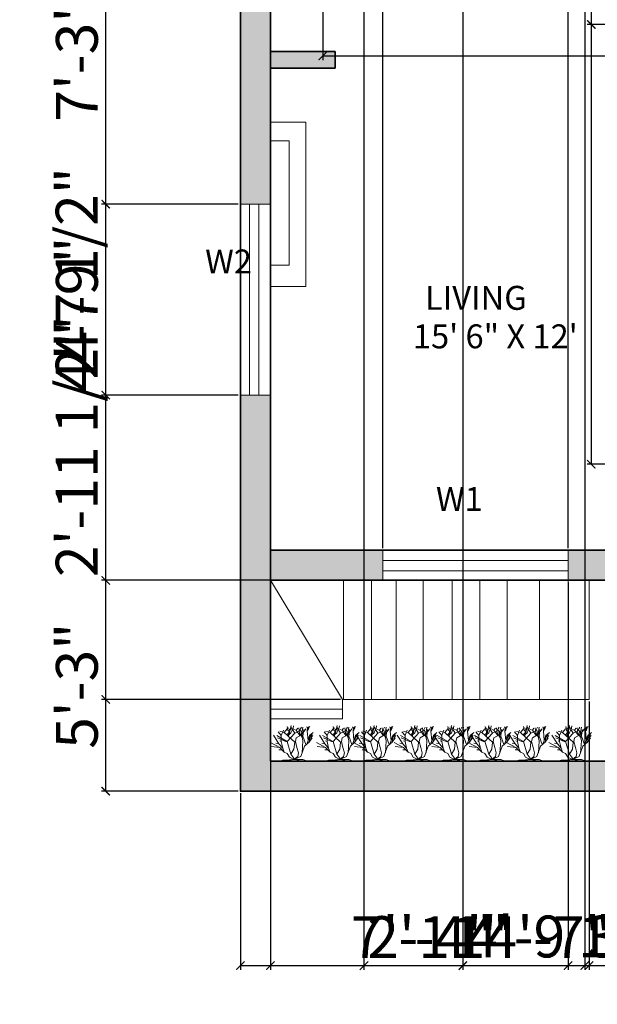
# Model space of a CAD drawing. Units: inches. Extents: x 1763 to 2368, y 1500 to 2097.
# Tile 1 of 24: x 1763 to 1936, y 1500 to 1794. Entities that reach past the tile are written whole.
import ezdxf

# ---------------------------------------------------------------- set-up
doc = ezdxf.new("R2010")
doc.units = ezdxf.units.IN
for name, color, linetype, lineweight in [('A-ANNO-DIMS', 2, 'Continuous', 18), ('A-ANNO-TEXT', 7, 'Continuous', 18), ('A-AREA-IDEN', 7, 'Continuous', 18), ('A-FLOR-STRS', 7, 'Continuous', 18), ('A-FURN', 8, 'Continuous', 18), ('A-WALL', 7, 'Continuous', 35), ('A-WALL-PATT', 7, 'Continuous', 13), ('trees', 3, 'Continuous', 13), ('windows', 1, 'Continuous', 18)]:
    doc.layers.add(name, color=color, linetype=linetype, lineweight=lineweight)
doc.styles.get("Standard").update_dxf_attribs({"font": 'arial.ttf'})
doc.dimstyles.new('ISO-25', dxfattribs={"dimtxt": 12.5, "dimasz": 2.5, "dimexe": 1.25, "dimexo": 0.625, "dimtad": 1, "dimdec": 0, "dimlunit": 4, "dimtxsty": 'Standard', "dimblk": 'ARCHTICK', "dimcen": 2.5, "dimclrd": 3, "dimclrt": 4, "dimadec": 0, "dimazin": 0, "dimtfac": 1, "dimtdec": 0, "dimtmove": 0, "dimatfit": 3, "dimfxl": 1, "dimarcsym": 0})

# ---------------------------------------------------------------- blocks, each defined once
blk = doc.blocks.new('*U17')
for p, q in [((-14.88, 18.24), (-17.76, 19.2)), ((-16.8, 16.32), (-15.36, 19.68)), ((-14.88, 18.24), (-12.96, 20.64)), ((-12.471, 19.775), (-12.898, 22.044)), ((-11.677, 19.071), (-12.471, 19.775)), ((-11.28, 19.619), (-12.104, 21.184)), ((-11.921, 18.836), (-10.64, 20.401)), ((-11.433, 18.289), (-10.457, 22.749)), ((-10.579, 18.054), (-9.846, 19.697)), ((-8.16, 17.76), (-10.56, 21.6)), ((-9.48, 19.775), (-8.992, 22.592)), ((-7.2, 19.68), (-8.64, 20.16)), ((-8.16, 17.76), (-5.28, 19.2)), ((-7.2, 19.68), (-6.24, 21.12)), ((-4.8, 16.32), (-7.2, 19.68)), ((-5.086, 17.741), (-5.513, 21.34)), ((-5.28, 19.2), (-3.84, 21.6)), ((-2.88, 12.96), (-4.32, 19.68)), ((-3.84, 16.8), (-0.96, 20.64)), ((-3.377, 18.602), (-2.888, 21.575)), ((-2.88, 15.84), (-2.4, 20.16)), ((-0.508, 21.888), (-0.081, 20.558)), ((-0.203, 19.149), (0.102, 21.34)), ((0.346, 13.203), (-0.203, 19.149)), ((-0.142, 19.384), (0.59, 20.401)), ((-0.02, 20.01), (0.896, 21.105)), ((0.041, 20.714), (1.384, 22.044)), ((0.102, 21.34), (0.835, 21.888)), ((-18.24, 11.04), (-21.755, 16.655)), ((-12.96, 12.48), (-19.68, 16.32)), ((-13.92, 12.48), (-19.2, 14.88)), ((-16.8, 16.32), (-18.72, 18.72)), ((-16.8, 12.48), (-17.76, 12.96)), ((-16.8, 12.48), (-16.8, 16.32)), ((-8.16, 12), (-14.88, 18.24)), ((-13.325, 16.724), (-11.433, 18.289)), ((-12.96, 12.48), (-8.16, 17.76)), ((-12.043, 15.628), (-11.921, 18.836)), ((-11.982, 16.802), (-10.579, 18.054)), ((-7.68, 12.48), (-7.2, 14.88)), ((-7.2, 14.88), (-3.84, 16.8)), ((-3.377, 15.315), (-5.086, 17.819)), ((-2.766, 16.802), (-3.377, 18.602)), ((-3.36, 5.28), (-2.88, 12.96)), ((-0.96, 10.56), (-2.88, 15.84)), ((-0.48, 10.8), (0.346, 13.203)), ((0.346, 13.203), (1.323, 16.254)), ((0.96, 12), (1.44, 15.36)), ((0.96, 12), (2.88, 14.88)), ((1.323, 16.254), (3.642, 18.289)), ((1.44, 15.36), (2.88, 17.28)), ((1.92, 13.44), (2.4, 15.36)), ((2.4, 15.36), (3.36, 16.32)), ((-17.76, 8.64), (-23.663, 11.961)), ((-17.76, 8.64), (-23.128, 9.222)), ((-18.24, 11.04), (-20.16, 11.52)), ((-15.84, 8.16), (-18.24, 11.04)), ((-16.32, 7.2), (-18.24, 7.2)), ((-14.88, 5.76), (-17.76, 8.64)), ((-15.84, 8.16), (-16.8, 12.48)), ((-14.88, 5.76), (-15.84, 8.16)), ((-12.96, 12.48), (-13.92, 12.48)), ((-10.56, 4.32), (-12.96, 12.48)), ((-10.56, 4.32), (-8.64, 7.68)), ((-8.64, 7.68), (-8.16, 12)), ((-6.72, 8.64), (-7.68, 12.48)), ((-5.76, 5.28), (-6.72, 8.64)), ((-4.32, 2.88), (-1.92, 9.6)), ((-1.92, 9.6), (0.96, 12)), ((-15.84, 0.48), (-17.76, 0)), ((-13.44, 0.48), (-15.84, 0.48)), ((-12.96, 4.8), (-14.88, 5.76)), ((-9.6, 0.96), (-13.44, 0.48)), ((-11.52, 2.4), (-12.96, 4.8)), ((-9.6, 0.96), (-12.96, 0)), ((-8.64, 0.96), (-11.52, 2.4)), ((-8.64, 1.92), (-10.56, 4.32)), ((-9.6, 0.96), (-7.68, 0.96)), ((-8.64, 0.96), (-4.32, 2.88)), ((-8.64, 0.96), (-6.24, 2.88)), ((-8.64, 0.96), (-8.64, 1.92)), ((-8.64, 0.96), (-2.88, 0.96)), ((-7.68, 0.96), (-6.24, 0.48)), ((-6.24, 2.88), (-5.76, 5.28)), ((-6.24, 0.48), (-3.36, 0)), ((-2.88, 0.96), (0, 0))]:
    blk.add_line(p, q)
blk = doc.blocks.new('_ArchTick')
at = {"color": 0, "linetype": 'ByBlock', "const_width": 0.15}
blk.add_lwpolyline([(-0.5, -0.5), (0.5, 0.5)], dxfattribs=at)
blk = doc.blocks.new('*D25')
at = {"layer": 'A-ANNO-DIMS', "color": 3, "lineweight": -2, "transparency": 16777216}
for p, q in [((1934.01, 1792.31), (1934.01, 1981.61)), ((1934.01, 1660.94), (1934.01, 1792.31))]:
    blk.add_line(p, q, dxfattribs=at)
at = {"layer": 'A-ANNO-DIMS', "color": 0, "lineweight": -2, "transparency": 16777216}
for p, q in [((1953.09, 1792.31), (1932.76, 1792.31)), ((1953.09, 1660.94), (1932.76, 1660.94))]:
    blk.add_line(p, q, dxfattribs=at)
at = {"layer": 'Defpoints', "color": 0, "transparency": 16777216}
for p in [(1934.01, 1792.31), (1953.72, 1792.31), (1953.72, 1660.94)]:
    blk.add_point(p, dxfattribs=at)
at = {"layer": 'A-ANNO-DIMS', "color": 3, "lineweight": -2, "transparency": 16777216, "xscale": 2.5, "yscale": 2.5, "zscale": 2.5}
for p, rotation in [((1934.01, 1792.31), 90), ((1934.01, 1660.94), 270)]:
    blk.add_blockref('_ArchTick', p, dxfattribs=dict(at, rotation=rotation))
at = {"layer": 'A-ANNO-DIMS', "color": 4, "transparency": 16777216, "insert": (1926.92, 1888.21), "char_height": 12.5, "attachment_point": 5, "rotation": 90}
blk.add_mtext('SECTIONAL 10\'-11 1/2"', dxfattribs=at)
blk = doc.blocks.new('*D27')
at = {"layer": 'A-ANNO-DIMS', "color": 0, "lineweight": -2, "transparency": 16777216}
for p, q in [((1853.71, 1795.96), (1853.71, 1781.68)), ((1944.71, 1795.96), (1944.71, 1781.68))]:
    blk.add_line(p, q, dxfattribs=at)
at = {"layer": 'A-ANNO-DIMS', "color": 3, "lineweight": -2, "transparency": 16777216}
for p, q in [((1853.71, 1782.93), (1944.71, 1782.93)), ((1944.71, 1782.93), (2085.85, 1782.93))]:
    blk.add_line(p, q, dxfattribs=at)
at = {"layer": 'Defpoints', "color": 0, "transparency": 16777216}
for p in [(1853.71, 1796.58), (1944.71, 1796.58), (1944.71, 1782.93)]:
    blk.add_point(p, dxfattribs=at)
at = {"layer": 'A-ANNO-DIMS', "color": 3, "lineweight": -2, "transparency": 16777216, "xscale": 2.5, "yscale": 2.5, "zscale": 2.5, "rotation": 180}
blk.add_blockref('_ArchTick', (1853.71, 1782.93), dxfattribs=at)
at = {"layer": 'A-ANNO-DIMS', "color": 3, "lineweight": -2, "transparency": 16777216, "xscale": 2.5, "yscale": 2.5, "zscale": 2.5}
blk.add_blockref('_ArchTick', (1944.71, 1782.93), dxfattribs=at)
at = {"layer": 'A-ANNO-DIMS', "color": 4, "transparency": 16777216, "insert": (2016.53, 1790.02), "char_height": 12.5, "attachment_point": 5}
blk.add_mtext('DINING SET 7\'-7"', dxfattribs=at)
blk = doc.blocks.new('*D39')
at = {"layer": 'A-ANNO-DIMS', "color": 0, "lineweight": -2, "transparency": 16777216}
for p, q in [((1829.09, 1562.65), (1829.09, 1509.91)), ((2003.86, 1562.65), (2003.86, 1509.91))]:
    blk.add_line(p, q, dxfattribs=at)
at = {"layer": 'A-ANNO-DIMS', "color": 3, "lineweight": -2, "transparency": 16777216}
blk.add_line((1829.09, 1511.16), (2003.86, 1511.16), dxfattribs=at)
at = {"layer": 'Defpoints', "color": 0, "transparency": 16777216}
for p in [(1829.09, 1563.27), (2003.86, 1563.27), (2003.86, 1511.16)]:
    blk.add_point(p, dxfattribs=at)
at = {"layer": 'A-ANNO-DIMS', "color": 3, "lineweight": -2, "transparency": 16777216, "xscale": 2.5, "yscale": 2.5, "zscale": 2.5, "rotation": 180}
blk.add_blockref('_ArchTick', (1829.09, 1511.16), dxfattribs=at)
at = {"layer": 'A-ANNO-DIMS', "color": 3, "lineweight": -2, "transparency": 16777216, "xscale": 2.5, "yscale": 2.5, "zscale": 2.5}
blk.add_blockref('_ArchTick', (2003.86, 1511.16), dxfattribs=at)
at = {"layer": 'A-ANNO-DIMS', "color": 4, "transparency": 16777216, "insert": (1916.48, 1518.06), "char_height": 12.5, "attachment_point": 5}
blk.add_mtext('14\'-7"', dxfattribs=at)
blk = doc.blocks.new('*D41')
at = {"layer": 'A-ANNO-DIMS', "color": 0, "lineweight": -2, "transparency": 16777216}
for p, q in [((1837.47, 1626.27), (1787.6, 1626.27)), ((1828.47, 1563.27), (1787.6, 1563.27))]:
    blk.add_line(p, q, dxfattribs=at)
at = {"layer": 'A-ANNO-DIMS', "color": 3, "lineweight": -2, "transparency": 16777216}
blk.add_line((1788.85, 1563.27), (1788.85, 1626.27), dxfattribs=at)
at = {"layer": 'Defpoints', "color": 0, "transparency": 16777216}
for p in [(1788.85, 1626.27), (1838.09, 1626.27), (1829.09, 1563.27)]:
    blk.add_point(p, dxfattribs=at)
at = {"layer": 'A-ANNO-DIMS', "color": 3, "lineweight": -2, "transparency": 16777216, "xscale": 2.5, "yscale": 2.5, "zscale": 2.5}
for p, rotation in [((1788.85, 1626.27), 90), ((1788.85, 1563.27), 270)]:
    blk.add_blockref('_ArchTick', p, dxfattribs=dict(at, rotation=rotation))
at = {"layer": 'A-ANNO-DIMS', "color": 4, "transparency": 16777216, "insert": (1781.84, 1594.77), "char_height": 12.5, "attachment_point": 5, "rotation": 90}
blk.add_mtext('5\'-3"', dxfattribs=at)
blk = doc.blocks.new('*D45')
at = {"layer": 'A-ANNO-DIMS', "color": 3, "lineweight": -2, "transparency": 16777216}
for p, q in [((1788.85, 1681.59), (1788.85, 1748.2)), ((1788.85, 1626.27), (1788.85, 1681.59))]:
    blk.add_line(p, q, dxfattribs=at)
at = {"layer": 'A-ANNO-DIMS', "color": 0, "lineweight": -2, "transparency": 16777216}
for p, q in [((1828.47, 1681.59), (1787.6, 1681.59)), ((1837.47, 1626.27), (1787.6, 1626.27))]:
    blk.add_line(p, q, dxfattribs=at)
at = {"layer": 'Defpoints', "color": 0, "transparency": 16777216}
for p in [(1788.85, 1681.59), (1829.09, 1681.59), (1838.09, 1626.27)]:
    blk.add_point(p, dxfattribs=at)
at = {"layer": 'A-ANNO-DIMS', "color": 3, "lineweight": -2, "transparency": 16777216, "xscale": 2.5, "yscale": 2.5, "zscale": 2.5}
for p, rotation in [((1788.85, 1681.59), 90), ((1788.85, 1626.27), 270)]:
    blk.add_blockref('_ArchTick', p, dxfattribs=dict(at, rotation=rotation))
at = {"layer": 'A-ANNO-DIMS', "color": 4, "transparency": 16777216, "insert": (1781.77, 1716.15), "char_height": 12.5, "attachment_point": 5, "rotation": 90}
blk.add_mtext('4\'-7 1/2"', dxfattribs=at)
blk = doc.blocks.new('*D46')
at = {"layer": 'A-ANNO-DIMS', "color": 0, "lineweight": -2, "transparency": 16777216}
for p, q in [((1828.47, 1738.64), (1787.6, 1738.64)), ((1828.47, 1681.59), (1787.6, 1681.59))]:
    blk.add_line(p, q, dxfattribs=at)
at = {"layer": 'A-ANNO-DIMS', "color": 3, "lineweight": -2, "transparency": 16777216}
blk.add_line((1788.85, 1681.59), (1788.85, 1738.64), dxfattribs=at)
at = {"layer": 'Defpoints', "color": 0, "transparency": 16777216}
for p in [(1788.85, 1738.64), (1829.09, 1738.64), (1829.09, 1681.59)]:
    blk.add_point(p, dxfattribs=at)
at = {"layer": 'A-ANNO-DIMS', "color": 3, "lineweight": -2, "transparency": 16777216, "xscale": 2.5, "yscale": 2.5, "zscale": 2.5}
for p, rotation in [((1788.85, 1738.64), 90), ((1788.85, 1681.59), 270)]:
    blk.add_blockref('_ArchTick', p, dxfattribs=dict(at, rotation=rotation))
at = {"layer": 'A-ANNO-DIMS', "color": 4, "transparency": 16777216, "insert": (1781.85, 1710.12), "char_height": 12.5, "attachment_point": 5, "rotation": 90}
blk.add_mtext('4\'-9"', dxfattribs=at)
blk = doc.blocks.new('*D47')
at = {"layer": 'A-ANNO-DIMS', "color": 0, "lineweight": -2, "transparency": 16777216}
for p, q in [((1828.47, 1825.59), (1787.6, 1825.59)), ((1828.47, 1738.64), (1787.6, 1738.64))]:
    blk.add_line(p, q, dxfattribs=at)
at = {"layer": 'A-ANNO-DIMS', "color": 3, "lineweight": -2, "transparency": 16777216}
blk.add_line((1788.85, 1738.64), (1788.85, 1825.59), dxfattribs=at)
at = {"layer": 'Defpoints', "color": 0, "transparency": 16777216}
for p in [(1788.85, 1825.59), (1829.09, 1825.59), (1829.09, 1738.64)]:
    blk.add_point(p, dxfattribs=at)
at = {"layer": 'A-ANNO-DIMS', "color": 3, "lineweight": -2, "transparency": 16777216, "xscale": 2.5, "yscale": 2.5, "zscale": 2.5}
for p, rotation in [((1788.85, 1825.59), 90), ((1788.85, 1738.64), 270)]:
    blk.add_blockref('_ArchTick', p, dxfattribs=dict(at, rotation=rotation))
at = {"layer": 'A-ANNO-DIMS', "color": 4, "transparency": 16777216, "insert": (1781.84, 1782.12), "char_height": 12.5, "attachment_point": 5, "rotation": 90}
blk.add_mtext('7\'-3"', dxfattribs=at)
blk = doc.blocks.new('*D57')
at = {"layer": 'A-ANNO-DIMS', "color": 0, "lineweight": -2, "transparency": 16777216}
for p, q in [((1927.07, 1625.65), (1927.07, 1509.91)), ((1990.09, 1625.65), (1990.09, 1509.91))]:
    blk.add_line(p, q, dxfattribs=at)
at = {"layer": 'A-ANNO-DIMS', "color": 3, "lineweight": -2, "transparency": 16777216}
blk.add_line((1927.07, 1511.16), (1990.09, 1511.16), dxfattribs=at)
at = {"layer": 'Defpoints', "color": 0, "transparency": 16777216}
for p in [(1927.07, 1626.27), (1990.09, 1626.27), (1990.09, 1511.16)]:
    blk.add_point(p, dxfattribs=at)
at = {"layer": 'A-ANNO-DIMS', "color": 3, "lineweight": -2, "transparency": 16777216, "xscale": 2.5, "yscale": 2.5, "zscale": 2.5, "rotation": 180}
blk.add_blockref('_ArchTick', (1927.07, 1511.16), dxfattribs=at)
at = {"layer": 'A-ANNO-DIMS', "color": 3, "lineweight": -2, "transparency": 16777216, "xscale": 2.5, "yscale": 2.5, "zscale": 2.5}
blk.add_blockref('_ArchTick', (1990.09, 1511.16), dxfattribs=at)
at = {"layer": 'A-ANNO-DIMS', "color": 4, "transparency": 16777216, "insert": (1958.58, 1518.17), "char_height": 12.5, "attachment_point": 5}
blk.add_mtext('5\'-3"', dxfattribs=at)
blk = doc.blocks.new('*D58')
at = {"layer": 'A-ANNO-DIMS', "color": 0, "lineweight": -2, "transparency": 16777216}
for p, q in [((1871.68, 1635.9), (1871.68, 2072.02)), ((1927.07, 1635.9), (1927.07, 2072.02))]:
    blk.add_line(p, q, dxfattribs=at)
at = {"layer": 'A-ANNO-DIMS', "color": 3, "lineweight": -2, "transparency": 16777216}
for p, q in [((1871.68, 2070.77), (1927.07, 2070.77)), ((1927.07, 2070.77), (1993.68, 2070.77))]:
    blk.add_line(p, q, dxfattribs=at)
at = {"layer": 'Defpoints', "color": 0, "transparency": 16777216}
for p in [(1927.07, 2070.77), (1871.68, 1635.27), (1927.07, 1635.27)]:
    blk.add_point(p, dxfattribs=at)
at = {"layer": 'A-ANNO-DIMS', "color": 3, "lineweight": -2, "transparency": 16777216, "xscale": 2.5, "yscale": 2.5, "zscale": 2.5, "rotation": 180}
blk.add_blockref('_ArchTick', (1871.68, 2070.77), dxfattribs=at)
at = {"layer": 'A-ANNO-DIMS', "color": 3, "lineweight": -2, "transparency": 16777216, "xscale": 2.5, "yscale": 2.5, "zscale": 2.5}
blk.add_blockref('_ArchTick', (1927.07, 2070.77), dxfattribs=at)
at = {"layer": 'A-ANNO-DIMS', "color": 4, "transparency": 16777216, "insert": (1961.63, 2077.86), "char_height": 12.5, "attachment_point": 5}
blk.add_mtext('4\'-7 1/2"', dxfattribs=at)
blk = doc.blocks.new('*D68')
at = {"layer": 'A-ANNO-DIMS', "color": 0, "lineweight": -2, "transparency": 16777216}
for p, q in [((1895.59, 1879.65), (1895.59, 1509.91)), ((1932.01, 1879.65), (1932.01, 1509.91))]:
    blk.add_line(p, q, dxfattribs=at)
at = {"layer": 'A-ANNO-DIMS', "color": 3, "lineweight": -2, "transparency": 16777216}
for p, q in [((1895.59, 1511.16), (1932.01, 1511.16)), ((1932.01, 1511.16), (1998.11, 1511.16))]:
    blk.add_line(p, q, dxfattribs=at)
at = {"layer": 'Defpoints', "color": 0, "transparency": 16777216}
for p in [(1895.59, 1880.27), (1932.01, 1880.27), (1932.01, 1511.16)]:
    blk.add_point(p, dxfattribs=at)
at = {"layer": 'A-ANNO-DIMS', "color": 3, "lineweight": -2, "transparency": 16777216, "xscale": 2.5, "yscale": 2.5, "zscale": 2.5, "rotation": 180}
blk.add_blockref('_ArchTick', (1895.59, 1511.16), dxfattribs=at)
at = {"layer": 'A-ANNO-DIMS', "color": 3, "lineweight": -2, "transparency": 16777216, "xscale": 2.5, "yscale": 2.5, "zscale": 2.5}
blk.add_blockref('_ArchTick', (1932.01, 1511.16), dxfattribs=at)
at = {"layer": 'A-ANNO-DIMS', "color": 4, "transparency": 16777216, "insert": (1966.31, 1518.25), "char_height": 12.5, "attachment_point": 5}
blk.add_mtext('3\'-0 1/2"', dxfattribs=at)
blk = doc.blocks.new('*D69')
at = {"layer": 'A-ANNO-DIMS', "color": 0, "lineweight": -2, "transparency": 16777216}
for p, q in [((1838.09, 1879.65), (1838.09, 1509.91)), ((1895.59, 1879.65), (1895.59, 1509.91))]:
    blk.add_line(p, q, dxfattribs=at)
at = {"layer": 'A-ANNO-DIMS', "color": 3, "lineweight": -2, "transparency": 16777216}
for p, q in [((1838.09, 1511.16), (1895.59, 1511.16)), ((1895.59, 1511.16), (1962.2, 1511.16))]:
    blk.add_line(p, q, dxfattribs=at)
at = {"layer": 'Defpoints', "color": 0, "transparency": 16777216}
for p in [(1838.09, 1880.27), (1895.59, 1880.27), (1895.59, 1511.16)]:
    blk.add_point(p, dxfattribs=at)
at = {"layer": 'A-ANNO-DIMS', "color": 3, "lineweight": -2, "transparency": 16777216, "xscale": 2.5, "yscale": 2.5, "zscale": 2.5, "rotation": 180}
blk.add_blockref('_ArchTick', (1838.09, 1511.16), dxfattribs=at)
at = {"layer": 'A-ANNO-DIMS', "color": 3, "lineweight": -2, "transparency": 16777216, "xscale": 2.5, "yscale": 2.5, "zscale": 2.5}
blk.add_blockref('_ArchTick', (1895.59, 1511.16), dxfattribs=at)
at = {"layer": 'A-ANNO-DIMS', "color": 4, "transparency": 16777216, "insert": (1930.15, 1518.24), "char_height": 12.5, "attachment_point": 5}
blk.add_mtext('4\'-9 1/2"', dxfattribs=at)
blk = doc.blocks.new('*D88')
at = {"layer": 'A-ANNO-DIMS', "color": 3, "lineweight": -2, "transparency": 16777216}
for p, q in [((1788.85, 1626.27), (1788.85, 1702.3)), ((1788.85, 1590.69), (1788.85, 1626.27))]:
    blk.add_line(p, q, dxfattribs=at)
at = {"layer": 'A-ANNO-DIMS', "color": 0, "lineweight": -2, "transparency": 16777216}
for p, q in [((1859.3, 1626.27), (1787.6, 1626.27)), ((1859, 1590.69), (1787.6, 1590.69))]:
    blk.add_line(p, q, dxfattribs=at)
at = {"layer": 'Defpoints', "color": 0, "transparency": 16777216}
for p in [(1788.85, 1626.27), (1859.93, 1626.27), (1859.62, 1590.69)]:
    blk.add_point(p, dxfattribs=at)
at = {"layer": 'A-ANNO-DIMS', "color": 3, "lineweight": -2, "transparency": 16777216, "xscale": 2.5, "yscale": 2.5, "zscale": 2.5}
for p, rotation in [((1788.85, 1626.27), 90), ((1788.85, 1590.69), 270)]:
    blk.add_blockref('_ArchTick', p, dxfattribs=dict(at, rotation=rotation))
at = {"layer": 'A-ANNO-DIMS', "color": 4, "transparency": 16777216, "insert": (1781.77, 1665.54), "char_height": 12.5, "attachment_point": 5, "rotation": 90}
blk.add_mtext('2\'-11 1/2"', dxfattribs=at)
blk = doc.blocks.new('*D89')
at = {"layer": 'A-ANNO-DIMS', "color": 0, "lineweight": -2, "transparency": 16777216}
for p, q in [((1933.33, 1590.06), (1933.33, 1509.91)), ((1838.09, 1584.21), (1838.09, 1509.91))]:
    blk.add_line(p, q, dxfattribs=at)
at = {"layer": 'A-ANNO-DIMS', "color": 3, "lineweight": -2, "transparency": 16777216}
blk.add_line((1838.09, 1511.16), (1933.33, 1511.16), dxfattribs=at)
at = {"layer": 'Defpoints', "color": 0, "transparency": 16777216}
for p in [(1933.33, 1590.69), (1838.09, 1584.84), (1933.33, 1511.16)]:
    blk.add_point(p, dxfattribs=at)
at = {"layer": 'A-ANNO-DIMS', "color": 3, "lineweight": -2, "transparency": 16777216, "xscale": 2.5, "yscale": 2.5, "zscale": 2.5, "rotation": 180}
blk.add_blockref('_ArchTick', (1838.09, 1511.16), dxfattribs=at)
at = {"layer": 'A-ANNO-DIMS', "color": 3, "lineweight": -2, "transparency": 16777216, "xscale": 2.5, "yscale": 2.5, "zscale": 2.5}
blk.add_blockref('_ArchTick', (1933.33, 1511.16), dxfattribs=at)
at = {"layer": 'A-ANNO-DIMS', "color": 4, "transparency": 16777216, "insert": (1885.71, 1518.06), "char_height": 12.5, "attachment_point": 5}
blk.add_mtext('7\'-11"', dxfattribs=at)
blk = doc.blocks.new('*D90')
at = {"layer": 'A-ANNO-DIMS', "color": 0, "lineweight": -2, "transparency": 16777216}
for p, q in [((1838.09, 1980.65), (1838.09, 1509.91)), ((1866.04, 1955.7), (1866.04, 1509.91))]:
    blk.add_line(p, q, dxfattribs=at)
at = {"layer": 'A-ANNO-DIMS', "color": 3, "lineweight": -2, "transparency": 16777216}
for p, q in [((1838.09, 1511.16), (1866.04, 1511.16)), ((1866.04, 1511.16), (1903.23, 1511.16))]:
    blk.add_line(p, q, dxfattribs=at)
at = {"layer": 'Defpoints', "color": 0, "transparency": 16777216}
for p in [(1838.09, 1981.27), (1866.04, 1956.32), (1866.04, 1511.16)]:
    blk.add_point(p, dxfattribs=at)
at = {"layer": 'A-ANNO-DIMS', "color": 3, "lineweight": -2, "transparency": 16777216, "xscale": 2.5, "yscale": 2.5, "zscale": 2.5, "rotation": 180}
blk.add_blockref('_ArchTick', (1838.09, 1511.16), dxfattribs=at)
at = {"layer": 'A-ANNO-DIMS', "color": 3, "lineweight": -2, "transparency": 16777216, "xscale": 2.5, "yscale": 2.5, "zscale": 2.5}
blk.add_blockref('_ArchTick', (1866.04, 1511.16), dxfattribs=at)
at = {"layer": 'A-ANNO-DIMS', "color": 4, "transparency": 16777216, "insert": (1885.88, 1518.06), "char_height": 12.5, "attachment_point": 5}
blk.add_mtext('2\'-4"', dxfattribs=at)

msp = doc.modelspace()

# ---------------------------------------------------------------- hatches: boundary and pattern name
at = {"layer": 'A-WALL-PATT'}
h = msp.add_hatch(color=256, dxfattribs=at)
h.dxf.hatch_style = 1
h.paths.add_polyline_path([(1838.09, 2034.27), (1838.09, 2043.27), (1829.09, 2043.27), (1829.09, 1953.39), (1838.09, 1953.39)])
h.paths.add_polyline_path([(1838.09, 1913.1), (1829.09, 1913.1), (1829.09, 1862.2), (1838.09, 1862.2)])
h.paths.add_polyline_path([(1838.09, 1825.59), (1829.09, 1825.59), (1829.09, 1738.64), (1838.09, 1738.64)])
h.paths.add_polyline_path([(1895.59, 1885.27), (1838.09, 1885.27), (1838.09, 1880.27), (1895.59, 1880.27)])
h.paths.add_polyline_path([(1857.39, 1784.27), (1838.09, 1784.27), (1838.09, 1779.27), (1857.39, 1779.27)])
h.paths.add_polyline_path([(1958.09, 1981.27), (1971.46, 1981.27), (1971.46, 1986.27), (1968.57, 1986.27), (1958.09, 1986.27), (1953.09, 1986.27), (1927.39, 1986.27), (1927.39, 1981.27), (1953.09, 1981.27), (1953.09, 1885.27), (1932.01, 1885.27), (1932.01, 1880.27), (1959.13, 1880.27), (1959.13, 1883.74), (1959.13, 1885.27), (1958.09, 1885.27)])
h.paths.add_polyline_path([(2018.09, 1981.27), (2031.02, 1981.27), (2031.02, 1986.27), (2018.09, 1986.27), (2013.09, 1986.27), (2001.23, 1986.27), (2001.23, 1981.27), (2013.09, 1981.27), (2013.09, 1885.27), (1982.18, 1885.27, -0.016629), (1982.23, 1883.74), (1982.23, 1880.27), (2049.69, 1880.27), (2049.69, 1883.74, -0.016629), (2049.74, 1885.27), (2018.09, 1885.27)])
h.paths.add_polyline_path([(2083.09, 1981.27), (2120.61, 1981.27), (2120.61, 1986.27), (2083.09, 1986.27), (2078.09, 1986.27), (2063.14, 1986.27), (2063.14, 1981.27), (2078.09, 1981.27), (2078.09, 1885.27), (2072.78, 1885.27), (2072.78, 1883.74), (2072.78, 1880.27), (2078.09, 1880.27), (2078.09, 1866.87), (2081.56, 1866.87, -0.016629), (2083.09, 1866.82)])
h.paths.add_polyline_path([(1871.68, 1635.27), (1838.09, 1635.27), (1838.09, 1626.27), (1871.68, 1626.27)], flags=17)
h.paths.add_polyline_path([(2100.58, 1688.27), (2060.09, 1688.27), (2060.09, 1679.27), (2100.58, 1679.27)], flags=17)
h.paths.add_polyline_path([(2180.09, 1688.27), (2148.74, 1688.27), (2148.74, 1679.27), (2180.09, 1679.27)], flags=17)
h.paths.add_polyline_path([(2189.09, 1746.22), (2180.09, 1746.22), (2180.09, 1743.42), (2180.12, 1743.42), (2180.12, 1726.72), (2180.09, 1572.27), (2034.91, 1572.27), (2034.91, 1565.6), (2034.91, 1563.27), (2189.09, 1563.27)])
h.paths.add_polyline_path([(2060.09, 1802.35, -0.016629), (2058.56, 1802.3), (2055.09, 1802.3), (2055.09, 1635.27), (2042.48, 1635.27), (2042.48, 1629.74), (2042.48, 1626.27), (2055.09, 1626.27), (2055.09, 1599.27), (2040.27, 1599.27), (2040.27, 1590.27), (2060.09, 1590.27)])
h.paths.add_polyline_path([(2019.39, 1629.74, -0.060569), (2020.06, 1635.27), (1995.09, 1635.27), (1990.09, 1635.27), (1927.07, 1635.27), (1927.07, 1626.27), (1990.09, 1626.27), (1990.09, 1590.27), (1995.09, 1590.27), (2005.2, 1590.27), (2005.2, 1599.27), (1995.09, 1599.27), (1995.09, 1626.27), (2019.39, 1626.27)])
edge = h.paths.add_edge_path()
edge.add_line((2180.09, 1837.27), (2167.2, 1837.27))
edge.add_spline(control_points=[(2167.2, 1837.27), (2167.19, 1837.27), (2167.18, 1837.27), (2167.18, 1837.27)], knot_values=[168.955493, 168.955493, 168.955493, 168.955493, 169.065871, 169.065871, 169.065871, 169.065871], degree=3, periodic=0)
edge.add_spline(control_points=[(2167.18, 1837.27), (2166.56, 1837.38), (2166.33, 1846.16), (2165.71, 1846.24)], knot_values=[159.864705, 159.864705, 159.864705, 159.864705, 168.955493, 168.955493, 168.955493, 168.955493], degree=3, periodic=0)
edge.add_line((2167.12, 1837.27), (2163.16, 1837.27))
edge.add_spline(control_points=[(2163.16, 1837.27), (2163.16, 1837.27), (2163.16, 1837.27), (2163.15, 1837.27)], knot_values=[150.537172, 150.537172, 150.537172, 150.537172, 150.553797, 150.553797, 150.553797, 150.553797], degree=3, periodic=0)
edge.add_spline(control_points=[(2163.15, 1837.27), (2162.29, 1837.29), (2161.59, 1846.23), (2160.88, 1846.24)], knot_values=[141.293426, 141.293426, 141.293426, 141.293426, 150.537172, 150.537172, 150.537172, 150.537172], degree=3, periodic=0)
edge.add_line((2163.08, 1837.27), (2158.7, 1837.27))
edge.add_spline(control_points=[(2158.7, 1837.27), (2158.7, 1837.27), (2158.7, 1837.27), (2158.7, 1837.27)], knot_values=[132.033544, 132.033544, 132.033544, 132.033544, 132.049151, 132.049151, 132.049151, 132.049151], degree=3, periodic=0)
edge.add_spline(control_points=[(2158.7, 1837.27), (2157.97, 1837.29), (2157.26, 1846.23), (2156.39, 1846.24)], knot_values=[122.786021, 122.786021, 122.786021, 122.786021, 132.033544, 132.033544, 132.033544, 132.033544], degree=3, periodic=0)
edge.add_line((2158.63, 1837.27), (2153.84, 1837.27))
edge.add_spline(control_points=[(2153.84, 1837.27), (2153.83, 1837.27), (2153.82, 1837.27), (2153.82, 1837.27)], knot_values=[113.451585, 113.451585, 113.451585, 113.451585, 113.562103, 113.562103, 113.562103, 113.562103], degree=3, periodic=0)
edge.add_spline(control_points=[(2153.82, 1837.27), (2153.17, 1837.38), (2152.88, 1846.19), (2152.4, 1846.24)], knot_values=[0, 0, 0, 0, 9.081854, 9.081854, 9.081854, 9.081854], degree=3, periodic=0)
edge.add_line((2153.76, 1837.27), (2150.39, 1837.27))
edge.add_spline(control_points=[(2150.39, 1837.27), (2150.38, 1837.27), (2150.37, 1837.27), (2150.36, 1837.27)], knot_values=[95.069382, 95.069382, 95.069382, 95.069382, 95.17519, 95.17519, 95.17519, 95.17519], degree=3, periodic=0)
edge.add_spline(control_points=[(2150.36, 1837.27), (2149.49, 1837.37), (2148.42, 1846.19), (2147.59, 1846.24)], knot_values=[85.824599, 85.824599, 85.824599, 85.824599, 95.069382, 95.069382, 95.069382, 95.069382], degree=3, periodic=0)
edge.add_line((2150.29, 1837.27), (2145.43, 1837.27))
edge.add_spline(control_points=[(2145.43, 1837.27), (2145.43, 1837.27), (2145.42, 1837.27), (2145.42, 1837.27)], knot_values=[76.505559, 76.505559, 76.505559, 76.505559, 76.547811, 76.547811, 76.547811, 76.547811], degree=3, periodic=0)
edge.add_spline(control_points=[(2145.42, 1837.27), (2144.68, 1837.31), (2143.8, 1846.19), (2142.95, 1846.24)], knot_values=[67.23945, 67.23945, 67.23945, 67.23945, 76.505559, 76.505559, 76.505559, 76.505559], degree=3, periodic=0)
edge.add_line((2145.35, 1837.27), (2134.57, 1837.27))
edge.add_spline(control_points=[(2134.57, 1837.27), (2134.57, 1837.27), (2134.56, 1837.27), (2134.56, 1837.27)], knot_values=[39.001463, 39.001463, 39.001463, 39.001463, 39.045107, 39.045107, 39.045107, 39.045107], degree=3, periodic=0)
edge.add_spline(control_points=[(2134.56, 1837.27), (2133.87, 1837.31), (2133.4, 1845.85), (2132.33, 1846.24)], knot_values=[29.79778, 29.79778, 29.79778, 29.79778, 39.001463, 39.001463, 39.001463, 39.001463], degree=3, periodic=0)
edge.add_line((2134.5, 1837.27), (2128.08, 1837.27))
edge.add_spline(control_points=[(2128.08, 1837.27), (2128.03, 1837.26), (2127.98, 1837.26), (2127.93, 1837.27)], knot_values=[19.482067, 19.482067, 19.482067, 19.482067, 19.869396, 19.869396, 19.869396, 19.869396], degree=3, periodic=0)
edge.add_spline(control_points=[(2125.01, 1846.24), (2126.16, 1844.66), (2126.82, 1837.57), (2127.93, 1837.27)], knot_values=[10.389805, 10.389805, 10.389805, 10.389805, 19.482067, 19.482067, 19.482067, 19.482067], degree=3, periodic=0)
edge.add_line((2127.93, 1837.27), (2083.09, 1837.27))
edge.add_line((2083.09, 1837.27), (2083.09, 1843.77))
edge.add_line((2083.09, 1843.77), (2081.56, 1843.77))
edge.add_line((2081.56, 1843.77), (2078.09, 1843.77))
edge.add_line((2078.09, 1843.77), (2078.09, 1837.27))
edge.add_line((2078.09, 1837.27), (2055.09, 1837.27))
edge.add_line((2055.09, 1837.27), (2055.09, 1825.4))
edge.add_line((2055.09, 1825.4), (2058.56, 1825.4))
edge.add_line((2058.56, 1825.4), (2060.09, 1825.4))
edge.add_line((2060.09, 1825.4), (2060.09, 1832.27))
edge.add_line((2060.09, 1832.27), (2122.44, 1832.27))
edge.add_spline(control_points=[(2122.44, 1832.27), (2122.73, 1832.58), (2123.01, 1832.62), (2123.28, 1832.27)], knot_values=[5.972033, 5.972033, 5.972033, 5.972033, 8.057258, 8.057258, 8.057258, 8.057258], degree=3, periodic=0)
edge.add_line((2123.28, 1832.27), (2137.95, 1832.27))
edge.add_spline(control_points=[(2137.95, 1832.27), (2137.96, 1832.27), (2137.97, 1832.27), (2137.98, 1832.27)], knot_values=[53.926862, 53.926862, 53.926862, 53.926862, 54.030075, 54.030075, 54.030075, 54.030075], degree=3, periodic=0)
edge.add_spline(control_points=[(2139.72, 1825.02), (2139.28, 1825.06), (2138.67, 1832.18), (2137.98, 1832.27)], knot_values=[54.030075, 54.030075, 54.030075, 54.030075, 61.445194, 61.445194, 61.445194, 61.445194], degree=3, periodic=0)
edge.add_line((2138.05, 1832.27), (2140.96, 1832.27))
edge.add_spline(control_points=[(2140.96, 1832.27), (2140.97, 1832.27), (2140.98, 1832.27), (2140.99, 1832.27)], knot_values=[68.854182, 68.854182, 68.854182, 68.854182, 68.971237, 68.971237, 68.971237, 68.971237], degree=3, periodic=0)
edge.add_spline(control_points=[(2143.19, 1825.02), (2142.44, 1825.07), (2141.56, 1832.16), (2140.99, 1832.27)], knot_values=[68.971237, 68.971237, 68.971237, 68.971237, 76.444911, 76.444911, 76.444911, 76.444911], degree=3, periodic=0)
edge.add_line((2141.04, 1832.27), (2145.43, 1832.27))
edge.add_spline(control_points=[(2145.43, 1832.27), (2145.44, 1832.27), (2145.45, 1832.27), (2145.46, 1832.27)], knot_values=[84.039047, 84.039047, 84.039047, 84.039047, 84.124041, 84.124041, 84.124041, 84.124041], degree=3, periodic=0)
edge.add_spline(control_points=[(2148.11, 1825.02), (2147.34, 1825.02), (2146.3, 1832.19), (2145.46, 1832.27)], knot_values=[84.124041, 84.124041, 84.124041, 84.124041, 91.773891, 91.773891, 91.773891, 91.773891], degree=3, periodic=0)
edge.add_line((2145.54, 1832.27), (2150.39, 1832.27))
edge.add_spline(control_points=[(2150.39, 1832.27), (2150.42, 1832.28), (2150.45, 1832.28), (2150.47, 1832.27)], knot_values=[99.381577, 99.381577, 99.381577, 99.381577, 99.573457, 99.573457, 99.573457, 99.573457], degree=3, periodic=0)
edge.add_spline(control_points=[(2153.97, 1825.02), (2153.09, 1825.28), (2151.53, 1832.1), (2150.47, 1832.27)], knot_values=[99.573457, 99.573457, 99.573457, 99.573457, 107.218357, 107.218357, 107.218357, 107.218357], degree=3, periodic=0)
edge.add_line((2150.57, 1832.27), (2155.6, 1832.27))
edge.add_spline(control_points=[(2155.6, 1832.27), (2155.6, 1832.27), (2155.61, 1832.27), (2155.62, 1832.27)], knot_values=[114.933058, 114.933058, 114.933058, 114.933058, 115.013624, 115.013624, 115.013624, 115.013624], degree=3, periodic=0)
edge.add_spline(control_points=[(2158.28, 1825.02), (2157.4, 1825.07), (2156.25, 1832.2), (2155.62, 1832.27)], knot_values=[115.013624, 115.013624, 115.013624, 115.013624, 122.616269, 122.616269, 122.616269, 122.616269], degree=3, periodic=0)
edge.add_line((2155.68, 1832.27), (2165.19, 1832.27))
edge.add_spline(control_points=[(2165.19, 1832.27), (2165.2, 1832.27), (2165.2, 1832.27), (2165.2, 1832.27)], knot_values=[145.488477, 145.488477, 145.488477, 145.488477, 145.516379, 145.516379, 145.516379, 145.516379], degree=3, periodic=0)
edge.add_spline(control_points=[(2167.45, 1825.02), (2166.96, 1825.02), (2166.06, 1832.25), (2165.2, 1832.27)], knot_values=[145.516379, 145.516379, 145.516379, 145.516379, 153.105469, 153.105469, 153.105469, 153.105469], degree=3, periodic=0)
edge.add_line((2165.29, 1832.27), (2168.93, 1832.27))
edge.add_spline(control_points=[(2168.93, 1832.27), (2168.98, 1832.29), (2169.04, 1832.29), (2169.1, 1832.27)], knot_values=[160.517439, 160.517439, 160.517439, 160.517439, 160.939723, 160.939723, 160.939723, 160.939723], degree=3, periodic=0)
edge.add_spline(control_points=[(2171.09, 1828.64), (2170.35, 1830.37), (2169.62, 1832.09), (2169.1, 1832.27)], knot_values=[160.939723, 160.939723, 160.939723, 160.939723, 164.738835, 164.738835, 164.738835, 164.738835], degree=3, periodic=0)
edge.add_line((2169.1, 1832.27), (2180.09, 1832.27))
edge.add_line((2180.09, 1832.27), (2180.09, 1837.27))
h.paths.add_polyline_path([(2189.09, 1885.52), (2180.09, 1885.52), (2180.09, 1813.32), (2180.12, 1813.32), (2180.12, 1796.62), (2180.12, 1795.26), (2189.09, 1795.26)])
h.paths.add_polyline_path([(2180.09, 1986.27), (2166.28, 1986.27), (2166.28, 1981.27), (2180.09, 1981.27)])
h.paths.add_polyline_path([(2189.09, 2043.27), (2180.09, 2043.27), (2180.09, 2034.27), (2180.09, 1934.11), (2189.09, 1934.11)])
h.paths.add_polyline_path([(1838.09, 1681.59), (1829.09, 1681.59), (1829.09, 1563.27), (2003.86, 1563.27), (2003.86, 1565.6), (2003.86, 1572.27), (1838.09, 1572.27)])

# ---------------------------------------------------------------- linework, layer by layer
at = {"layer": 'A-FLOR-STRS'}
for p, q in [((1859.62, 1590.69), (1838.09, 1626.27)), ((1859.93, 1626.27), (1859.93, 1590.69)), ((1868.29, 1626.27), (1868.29, 1590.69)), ((1875.64, 1626.27), (1875.64, 1590.69)), ((1883.74, 1626.27), (1883.74, 1590.69)), ((1892.36, 1626.27), (1892.36, 1590.69)), ((1900.72, 1626.27), (1900.72, 1590.69)), ((1908.83, 1626.27), (1908.83, 1590.69)), ((1918.46, 1626.27), (1918.46, 1590.69)), ((1927.07, 1626.27), (1927.07, 1590.69)), ((1933.33, 1626.27), (1933.33, 1590.69)), ((1933.33, 1590.69), (1859.62, 1590.69)), ((1859.62, 1590.69), (1859.62, 1584.84)), ((1859.62, 1587.76), (1838.09, 1587.76)), ((1859.62, 1584.84), (1838.09, 1584.84))]:
    msp.add_line(p, q, dxfattribs=at)
at = {"layer": 'A-FURN'}
for points in [[(1838.09, 1763.11), (1848.67, 1763.11), (1848.67, 1714.08), (1838.09, 1714.08)], [(1838.09, 1757.61), (1843.68, 1757.61), (1843.68, 1720.46), (1838.09, 1720.46)]]:
    msp.add_lwpolyline(points, close=True, dxfattribs=at)
at = {"layer": 'A-WALL'}
for p, q in [((1838.09, 1572.27), (1838.09, 2034.27)), ((1838.09, 1784.27), (1857.39, 1784.27)), ((1857.39, 1784.27), (1857.39, 1779.27)), ((1838.09, 1779.27), (1857.39, 1779.27)), ((1838.09, 1635.27), (1990.09, 1635.27)), ((1838.09, 1626.27), (1990.09, 1626.27)), ((2004.54, 1572.27), (1838.09, 1572.27))]:
    msp.add_line(p, q, dxfattribs=at)
msp.add_lwpolyline([(2003.86, 1563.27), (1829.09, 1563.27), (1829.09, 2043.27), (2189.09, 2043.27), (2189.09, 1563.27), (2034.91, 1563.27)], dxfattribs=at)
at = {"layer": 'windows'}
for p, q in [((1838.09, 1738.64), (1829.09, 1738.64)), ((1829.09, 1738.64), (1829.09, 1681.59)), ((1831.78, 1681.59), (1831.78, 1738.64)), ((1834.64, 1681.59), (1834.64, 1738.64)), ((1838.09, 1681.59), (1838.09, 1738.64)), ((1829.09, 1681.59), (1838.09, 1681.59)), ((1871.68, 1635.27), (1871.68, 1626.27)), ((1927.07, 1635.27), (1871.68, 1635.27)), ((1927.07, 1626.27), (1927.07, 1635.27)), ((1871.68, 1632.21), (1927.07, 1632.21)), ((1871.68, 1629.13), (1927.07, 1629.13)), ((1871.68, 1626.27), (1927.07, 1626.27))]:
    msp.add_line(p, q, dxfattribs=at)

# ---------------------------------------------------------------- block references
at = {"layer": 'trees', "xscale": 0.4676307550764569, "yscale": 0.4676307550764569, "zscale": 0.4676307550764569}
for p in [(1849.16, 1572.27), (1862.88, 1572.27), (1874.01, 1572.27), (1886.16, 1572.27), (1897.13, 1572.27), (1908.27, 1572.27), (1908.27, 1572.27), (1919.75, 1572.27), (1932.38, 1572.27)]:
    msp.add_blockref('*U17', p, dxfattribs=at)

# ---------------------------------------------------------------- texts
at = {"layer": 'A-ANNO-TEXT'}
for s, p in [('W2', (1818.57, 1717.94)), ('W1', (1887.55, 1646.99))]:
    msp.add_text(s, height=7.155, dxfattribs=at).set_placement(p)
at = {"layer": 'A-AREA-IDEN'}
for s, height, p in [('LIVING', 7.155, (1884.27, 1707.08)), ('15\' 6" X 12\'', 7.1545, (1880.66, 1695.58))]:
    msp.add_text(s, height=height, dxfattribs=at).set_placement(p)

# ---------------------------------------------------------------- dimensions: what is measured, and where the dimension line sits
at = {"layer": 'A-ANNO-DIMS'}
for base, p1, p2, picture, middle in [((1927.07, 2070.77), (1871.68, 1635.27), (1927.07, 1635.27), '*D58', (1961.63, 2077.86)), ((1866.0388, 1511.1561), (1838.0918, 1981.2727), (1866.0388, 1956.3234), '*D90', (1885.8845, 1518.0567)), ((1895.59, 1511.16), (1838.09, 1880.27), (1895.59, 1880.27), '*D69', (1930.15, 1518.24)), ((1932.01, 1511.16), (1895.59, 1880.27), (1932.01, 1880.27), '*D68', (1966.31, 1518.25)), ((1990.09, 1511.16), (1927.07, 1626.27), (1990.09, 1626.27), '*D57', (1958.58, 1518.17)), ((1933.33, 1511.16), (1838.09, 1584.84), (1933.33, 1590.69), '*D89', (1885.71, 1518.06)), ((2003.86, 1511.16), (1829.09, 1563.27), (2003.86, 1563.27), '*D39', (1916.48, 1518.06))]:
    dim = msp.add_linear_dim(base=base, p1=p1, p2=p2, dimstyle='ISO-25', override={"dimdec": 1, "dimlfac": 1, "dimrnd": 0, "dimzin": 1, "dimdsep": 46, "dimlunit": 4, "dimfrac": 2}, dxfattribs=at)
    dim.commit()
    dim.dimension.update_dxf_attribs({"geometry": picture, "text_midpoint": middle})
dim = msp.add_linear_dim(base=(1934.01, 1792.31), p1=(1953.72, 1660.94), p2=(1953.72, 1792.31), angle=90, text='SECTIONAL <>', dimstyle='ISO-25', override={"dimdec": 1, "dimlfac": 1, "dimrnd": 0, "dimzin": 1, "dimdsep": 46, "dimlunit": 4, "dimfrac": 2}, dxfattribs=at)
dim.commit()
dim.dimension.update_dxf_attribs({"geometry": '*D25', "text_midpoint": (1926.92, 1888.21)})
for base, p1, p2, picture, middle in [((1788.8549, 1825.5896), (1829.0918, 1738.6434), (1829.0918, 1825.5896), '*D47', (1781.8435, 1782.1165)), ((1788.85, 1681.59), (1838.09, 1626.27), (1829.09, 1681.59), '*D45', (1781.77, 1716.15)), ((1788.8549, 1738.6434), (1829.0918, 1681.5919), (1829.0918, 1738.6434), '*D46', (1781.8478, 1710.1176)), ((1788.85, 1626.27), (1859.62, 1590.69), (1859.93, 1626.27), '*D88', (1781.77, 1665.54)), ((1788.85, 1626.27), (1829.09, 1563.27), (1838.09, 1626.27), '*D41', (1781.84, 1594.77))]:
    dim = msp.add_linear_dim(base=base, p1=p1, p2=p2, angle=90, dimstyle='ISO-25', override={"dimdec": 1, "dimlfac": 1, "dimrnd": 0, "dimzin": 1, "dimdsep": 46, "dimlunit": 4, "dimfrac": 2}, dxfattribs=at)
    dim.commit()
    dim.dimension.update_dxf_attribs({"geometry": picture, "text_midpoint": middle})
dim = msp.add_linear_dim(base=(1944.71, 1782.93), p1=(1853.71, 1796.58), p2=(1944.71, 1796.58), text='DINING SET <>', dimstyle='ISO-25', override={"dimdec": 1, "dimlfac": 1, "dimrnd": 0, "dimzin": 1, "dimdsep": 46, "dimlunit": 4, "dimfrac": 2}, dxfattribs=at)
dim.commit()
dim.dimension.update_dxf_attribs({"geometry": '*D27', "text_midpoint": (2016.53, 1790.02)})

doc.saveas('drawing.dxf')
